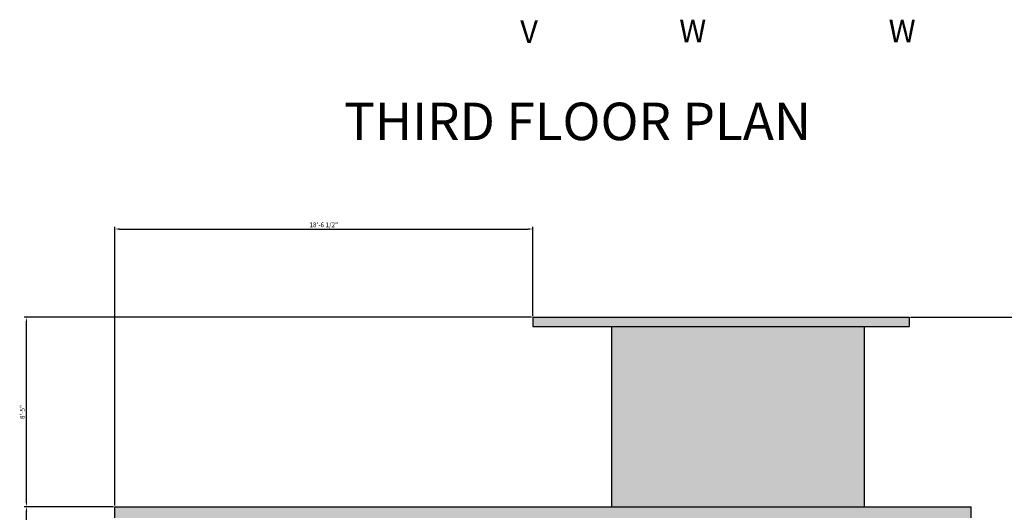
# Model space of a CAD drawing. Units: inches. Extents: x 2391 to 16591, y 7259 to 10239.
# Tile 10 of 27: x 2963 to 3487, y 8236 to 8498. Entities that reach past the tile are written whole.
import ezdxf

# ---------------------------------------------------------------- set-up
doc = ezdxf.new("R2010")
doc.units = ezdxf.units.IN
for name, color, linetype, lineweight in [('A-ANNO-DIMS', 4, 'Continuous', 18), ('A-ANNO-IDEN', 2, 'Continuous', 18), ('A-ANNO-TITL', 3, 'Continuous', 30), ('A-ELEV', 7, 'Continuous', 30), ('A-ELEV-SURF-PATT', 253, 'Continuous', 13), ('A-ROOF', 7, 'Continuous', 25)]:
    doc.layers.add(name, color=color, linetype=linetype, lineweight=lineweight)
doc.styles.get("Standard").update_dxf_attribs({"font": 'arial.ttf'})
doc.dimstyles.new('ISO-25', dxfattribs={"dimtxt": 2.5, "dimasz": 2.5, "dimexe": 1.25, "dimexo": 0.625, "dimtad": 1, "dimdec": 0, "dimlunit": 3, "dimtxsty": 'Standard', "dimcen": 2.5, "dimadec": 0, "dimazin": 0, "dimtfac": 1, "dimtdec": 0, "dimtmove": 0, "dimatfit": 3, "dimfxl": 1, "dimarcsym": 0})

# ---------------------------------------------------------------- blocks, each defined once
blk = doc.blocks.new('*D84')
at = {"layer": 'A-ANNO-DIMS', "color": 0, "lineweight": -2, "transparency": 16777216}
for p, q in [((3437.4, 8339.52), (3518.08, 8339.52)), ((3516.83, 7579.02), (3516.83, 8337.02)), ((3464.4, 7576.52), (3518.08, 7576.52))]:
    blk.add_line(p, q, dxfattribs=at)
at = {"layer": 'A-ANNO-DIMS', "color": 0, "transparency": 16777216}
for points in [[(3516.41, 8337.02), (3517.24, 8337.02), (3516.83, 8339.52)], [(3516.41, 7579.02), (3517.24, 7579.02), (3516.83, 7576.52)]]:
    blk.add_solid(points, dxfattribs=at)
at = {"layer": 'Defpoints', "color": 0, "transparency": 16777216}
for p in [(3436.78, 8339.52), (3516.83, 8339.52), (3463.78, 7576.52)]:
    blk.add_point(p, dxfattribs=at)
at = {"layer": 'A-ANNO-DIMS', "color": 0, "transparency": 16777216, "insert": (3514.93, 7958.02), "char_height": 2.5, "attachment_point": 5, "rotation": 90}
blk.add_mtext('63\'-7"', dxfattribs=at)
blk = doc.blocks.new('*D88')
at = {"layer": 'A-ANNO-DIMS', "color": 0, "lineweight": -2, "transparency": 16777216}
for p, q in [((3013.15, 8238.52), (2965.48, 8238.52)), ((2966.73, 8079.02), (2966.73, 8236.02)), ((3013.15, 8076.52), (2965.48, 8076.52))]:
    blk.add_line(p, q, dxfattribs=at)
at = {"layer": 'A-ANNO-DIMS', "color": 0, "transparency": 16777216}
for points in [[(2966.31, 8236.02), (2967.14, 8236.02), (2966.73, 8238.52)], [(2966.31, 8079.02), (2967.14, 8079.02), (2966.73, 8076.52)]]:
    blk.add_solid(points, dxfattribs=at)
at = {"layer": 'Defpoints', "color": 0, "transparency": 16777216}
for p in [(2966.73, 8238.52), (3013.78, 8238.52), (3013.78, 8076.52)]:
    blk.add_point(p, dxfattribs=at)
at = {"layer": 'A-ANNO-DIMS', "color": 0, "transparency": 16777216, "insert": (2964.83, 8157.52), "char_height": 2.5, "attachment_point": 5, "rotation": 90}
blk.add_mtext('13\'-6"', dxfattribs=at)
blk = doc.blocks.new('*D89')
at = {"layer": 'A-ANNO-DIMS', "color": 0, "lineweight": -2, "transparency": 16777216}
for p, q in [((3235.65, 8339.52), (2965.48, 8339.52)), ((2966.73, 8241.02), (2966.73, 8337.02)), ((3013.15, 8238.52), (2965.48, 8238.52))]:
    blk.add_line(p, q, dxfattribs=at)
at = {"layer": 'A-ANNO-DIMS', "color": 0, "transparency": 16777216}
for points in [[(2966.31, 8337.02), (2967.14, 8337.02), (2966.73, 8339.52)], [(2966.31, 8241.02), (2967.14, 8241.02), (2966.73, 8238.52)]]:
    blk.add_solid(points, dxfattribs=at)
at = {"layer": 'Defpoints', "color": 0, "transparency": 16777216}
for p in [(2966.73, 8339.52), (3236.28, 8339.52), (3013.78, 8238.52)]:
    blk.add_point(p, dxfattribs=at)
at = {"layer": 'A-ANNO-DIMS', "color": 0, "transparency": 16777216, "insert": (2964.83, 8289.02), "char_height": 2.5, "attachment_point": 5, "rotation": 90}
blk.add_mtext('8\'-5"', dxfattribs=at)
blk = doc.blocks.new('*D90')
at = {"layer": 'A-ANNO-DIMS', "color": 0, "lineweight": -2, "transparency": 16777216}
for p, q in [((3013.78, 8239.14), (3013.78, 8387.82)), ((3016.28, 8386.57), (3233.78, 8386.57)), ((3236.28, 8340.14), (3236.28, 8387.82))]:
    blk.add_line(p, q, dxfattribs=at)
at = {"layer": 'A-ANNO-DIMS', "color": 0, "transparency": 16777216}
for points in [[(3016.28, 8386.99), (3016.28, 8386.15), (3013.78, 8386.57)], [(3233.78, 8386.99), (3233.78, 8386.15), (3236.28, 8386.57)]]:
    blk.add_solid(points, dxfattribs=at)
at = {"layer": 'Defpoints', "color": 0, "transparency": 16777216}
for p in [(3236.28, 8386.57), (3236.28, 8339.52), (3013.78, 8238.52)]:
    blk.add_point(p, dxfattribs=at)
at = {"layer": 'A-ANNO-DIMS', "color": 0, "transparency": 16777216, "insert": (3125.03, 8388.49), "char_height": 2.5, "attachment_point": 5}
blk.add_mtext('18\'-6 1/2"', dxfattribs=at)

msp = doc.modelspace()

# ---------------------------------------------------------------- hatches: boundary and pattern name
at = {"layer": 'A-ELEV-SURF-PATT'}
h = msp.add_hatch(color=256, dxfattribs=at)
h.dxf.hatch_style = 1
h.paths.add_polyline_path([(3469.78, 7746.52), (3469.78, 7752.52), (3013.78, 7752.52), (3013.78, 7746.52)])
h.paths.add_polyline_path([(3469.78, 7908.52), (3469.78, 7914.52), (3013.78, 7914.52), (3013.78, 7908.52)])
h.paths.add_polyline_path([(3469.78, 8070.52), (3469.78, 8076.52), (3013.78, 8076.52), (3013.78, 8070.52)])
h.paths.add_polyline_path([(3013.78, 8238.52), (3013.78, 8232.52), (3469.78, 8232.52), (3469.78, 8238.52)])
h.paths.add_polyline_path([(3236.28, 8339.52), (3236.28, 8334.52), (3436.78, 8334.52), (3436.78, 8339.52)])
h = msp.add_hatch(color=256, dxfattribs=at)
h.dxf.hatch_style = 1
h.paths.add_polyline_path([(3278.28, 8334.52), (3278.28, 8238.52), (3412.78, 8238.52), (3412.78, 8334.52)])

# ---------------------------------------------------------------- linework, layer by layer
at = {"layer": 'A-ELEV'}
for p, q in [((3013.78, 8232.52), (3013.78, 8238.52)), ((3469.78, 8232.52), (3469.78, 8238.52))]:
    msp.add_line(p, q, dxfattribs=at)
at = {"layer": 'A-ROOF'}
for p, q in [((3236.28, 8339.52), (3436.78, 8339.52)), ((3236.28, 8339.52), (3236.28, 8334.52)), ((3436.78, 8339.52), (3436.78, 8334.52)), ((3236.28, 8334.52), (3436.78, 8334.52)), ((3278.28, 8334.52), (3278.28, 8238.52)), ((3412.78, 8334.52), (3412.78, 8238.52)), ((3013.78, 8238.52), (3469.78, 8238.52))]:
    msp.add_line(p, q, dxfattribs=at)

# ---------------------------------------------------------------- texts
at = {"layer": 'A-ANNO-IDEN', "char_height": 12, "attachment_point": 1}
for s, width, insert in [('V', 46.245, (3229.64, 8497.84)), ('W', 47.6363, (3314.32, 8498.2)), ('W', 38.8857, (3425.82, 8498.14))]:
    msp.add_mtext_dynamic_manual_height_columns(s, width=width, gutter_width=12.5, heights=[0], dxfattribs=dict(at, insert=insert))
at = {"layer": 'A-ANNO-TITL', "insert": (3135.86, 8453.96), "char_height": 20, "attachment_point": 1}
msp.add_mtext_dynamic_manual_height_columns('THIRD FLOOR PLAN', width=567.8276, gutter_width=12.5, heights=[0], dxfattribs=at)

# ---------------------------------------------------------------- dimensions: what is measured, and where the dimension line sits
at = {"layer": 'A-ANNO-DIMS'}
dim = msp.add_linear_dim(base=(3236.28, 8386.57), p1=(3013.78, 8238.52), p2=(3236.28, 8339.52), dimstyle='ISO-25', override={"dimdec": 1, "dimlfac": 1, "dimrnd": 0, "dimzin": 1, "dimdsep": 46, "dimlunit": 4, "dimfrac": 2}, dxfattribs=at)
dim.commit()
dim.dimension.update_dxf_attribs({"geometry": '*D90', "text_midpoint": (3125.03, 8388.49)})
for base, p1, p2, picture, middle in [((2966.73, 8339.52), (3013.78, 8238.52), (3236.28, 8339.52), '*D89', (2964.83, 8289.02)), ((3516.83, 8339.52), (3463.78, 7576.52), (3436.78, 8339.52), '*D84', (3514.93, 7958.02)), ((2966.73, 8238.52), (3013.78, 8076.52), (3013.78, 8238.52), '*D88', (2964.83, 8157.52))]:
    dim = msp.add_linear_dim(base=base, p1=p1, p2=p2, angle=90, dimstyle='ISO-25', override={"dimdec": 1, "dimlfac": 1, "dimrnd": 0, "dimzin": 1, "dimdsep": 46, "dimlunit": 4, "dimfrac": 2}, dxfattribs=at)
    dim.commit()
    dim.dimension.update_dxf_attribs({"geometry": picture, "text_midpoint": middle})

doc.saveas('drawing.dxf')
